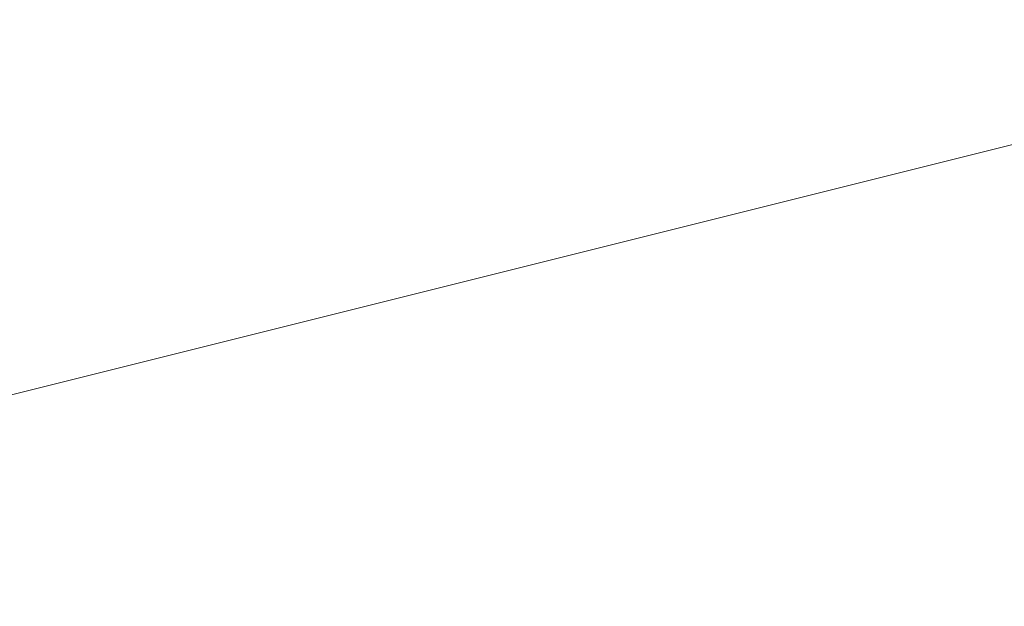
# Model space of a CAD drawing. Units: inches. Extents: x 2091 to 2899, y 967 to 2217.
# Tile 101 of 256: x 2252.3817 to 2252.951, y 1100.0709 to 1100.4099. Entities that reach past the tile are written whole.
import ezdxf

# ---------------------------------------------------------------- set-up
doc = ezdxf.new("R2010")
doc.units = ezdxf.units.IN
doc.layers.add('A-ANNO-DIMS', color=2, linetype='Continuous', lineweight=18)
doc.layers.add('L-PLNT-TREE', color=94, linetype='Continuous', lineweight=13)
doc.layers.add('A-WALL-PATT', color=141, linetype='Continuous', lineweight=13, true_color=0xadddf7)
doc.styles.get("Standard").update_dxf_attribs({"font": 'arial.ttf'})
doc.dimstyles.new('ISO-25', dxfattribs={"dimtxt": 4, "dimasz": 4, "dimexe": 1.25, "dimexo": 0.625, "dimtad": 1, "dimdec": 0, "dimlunit": 3, "dimtxsty": 'Standard', "dimcen": 2.5, "dimadec": 0, "dimazin": 0, "dimtfac": 1, "dimtdec": 0, "dimtmove": 0, "dimatfit": 3, "dimfxl": 1, "dimarcsym": 0})

# ---------------------------------------------------------------- blocks, each defined once
blk = doc.blocks.new('*U29')
blk.add_line((-402.336, 12.192), (-451.104, 0))
blk = doc.blocks.new('*D71')
at = {"layer": 'A-ANNO-DIMS', "color": 0, "lineweight": -2, "transparency": 16777216}
for p, q in [((2212.1436, 1351.29406), (2212.1436, 969.4643)), ((2452.1436, 1351.29406), (2452.1436, 969.4643)), ((2216.1436, 970.7143), (2448.1436, 970.7143))]:
    blk.add_line(p, q, dxfattribs=at)
at = {"layer": 'A-ANNO-DIMS', "color": 0, "transparency": 16777216}
for points in [[(2216.1436, 971.38097), (2216.1436, 970.04764), (2212.1436, 970.7143)], [(2448.1436, 971.38097), (2448.1436, 970.04764), (2452.1436, 970.7143)]]:
    blk.add_solid(points, dxfattribs=at)
at = {"layer": 'Defpoints', "color": 0, "transparency": 16777216}
for p in [(2212.1436, 1351.91906), (2452.1436, 1351.91906), (2452.1436, 970.7143)]:
    blk.add_point(p, dxfattribs=at)
at = {"layer": 'A-ANNO-DIMS', "color": 0, "transparency": 16777216, "insert": (2332.1436, 973.38159), "char_height": 4, "attachment_point": 5}
blk.add_mtext('20\'-0"', dxfattribs=at)
blk = doc.blocks.new('*D75')
at = {"layer": 'A-ANNO-DIMS', "color": 0, "lineweight": -2, "transparency": 16777216}
for p, q in [((2212.1436, 1274.79406), (2212.1436, 969.4643)), ((2308.1436, 1274.79406), (2308.1436, 969.4643)), ((2216.1436, 970.7143), (2304.1436, 970.7143))]:
    blk.add_line(p, q, dxfattribs=at)
at = {"layer": 'A-ANNO-DIMS', "color": 0, "transparency": 16777216}
for points in [[(2216.1436, 971.38097), (2216.1436, 970.04764), (2212.1436, 970.7143)], [(2304.1436, 971.38097), (2304.1436, 970.04764), (2308.1436, 970.7143)]]:
    blk.add_solid(points, dxfattribs=at)
at = {"layer": 'Defpoints', "color": 0, "transparency": 16777216}
for p in [(2212.1436, 1275.41906), (2308.1436, 1275.41906), (2308.1436, 970.7143)]:
    blk.add_point(p, dxfattribs=at)
at = {"layer": 'A-ANNO-DIMS', "color": 0, "transparency": 16777216, "insert": (2260.1436, 973.38159), "char_height": 4, "attachment_point": 5}
blk.add_mtext('8\'-0"', dxfattribs=at)

msp = doc.modelspace()

# ---------------------------------------------------------------- hatches: boundary and pattern name
at = {"layer": 'A-WALL-PATT'}
h = msp.add_hatch(color=256, dxfattribs=at)
h.dxf.hatch_style = 1
h.paths.add_polyline_path([(2803.1436, 2050.91906), (2203.1436, 2050.91906), (2203.1436, 1090.91906), (2803.1436, 1090.91906)])
h.paths.add_polyline_path([(2635.79885, 1147.54046), (2674.52405, 1147.54046, 0.376086), (2678.52967, 1152.8802), (2678.52967, 1159.55647, 0.333335), (2674.52432, 1163.56185), (2674.52432, 1163.56185), (2674.52432, 1192.93439), (2635.80597, 1192.93439), (2597.08762, 1192.93439), (2597.08762, 1163.56185, 0.333335), (2593.08228, 1159.55647), (2593.08228, 1152.8802, 0.376086), (2597.08789, 1147.54046)], flags=0)
h.paths.add_polyline_path([(2436.01043, 1278.24078, 0.000483), (2435.95264, 1278.21503, -0.001328), (2435.93563, 1278.11169, -0.001711), (2436.11644, 1278.04076, 0.002185)], flags=0)
h.paths.add_polyline_path([(2794.1436, 1143.41906), (2794.1436, 1347.41906), (2543.37017, 1347.41906), (2543.37017, 1351.91906), (2794.1436, 1351.91906), (2794.1436, 1392.71355), (2793.9474, 1392.71355), (2793.9474, 1473.5369), (2794.1436, 1473.5369), (2794.1436, 1531.91906), (2650.1436, 1531.91906), (2650.1436, 1536.41906), (2794.1436, 1536.41906), (2794.1436, 1692.41906), (2609.37561, 1692.41906), (2609.37561, 1644.41906), (2604.87561, 1644.41906), (2604.87561, 1744.91906), (2609.37561, 1744.91906), (2609.37561, 1696.91906), (2794.1436, 1696.91906), (2794.1436, 1780.91906), (2609.6436, 1780.91906), (2493.87561, 1780.91906), (2493.87561, 1785.41906), (2609.6436, 1785.41906), (2794.1436, 1785.41906), (2794.1436, 1847.93882), (2793.95122, 1847.93882), (2793.95122, 1928.76217), (2794.1436, 1928.76217), (2794.1436, 1941.41906), (2614.1436, 1941.41906), (2614.1436, 1821.41906), (2609.6436, 1821.41906), (2609.6436, 1941.41906), (2392.1436, 1941.41906), (2392.1436, 1819.91906), (2387.6436, 1819.91906), (2387.6436, 1941.41906), (2212.1436, 1941.41906), (2212.1436, 1783.91906), (2392.1436, 1783.91906), (2392.1436, 1780.91906), (2212.1436, 1780.91906), (2212.1436, 1629.41906), (2387.6436, 1629.41906), (2387.6436, 1744.91906), (2392.1436, 1744.91906), (2392.1436, 1627.91906), (2317.1436, 1627.91906), (2317.1436, 1551.41906), (2317.1436, 1536.41906), (2459.38359, 1536.41906), (2459.38359, 1602.39648), (2463.88359, 1602.39648), (2463.88359, 1531.91906), (2456.6436, 1531.91906), (2456.6436, 1529.91906), (2452.1436, 1529.91906), (2452.1436, 1531.91906), (2312.6436, 1531.91906), (2312.6436, 1551.41906), (2306.1436, 1551.41906), (2306.1436, 1555.91906), (2308.1436, 1555.91906), (2308.1436, 1551.41906), (2312.6436, 1551.41906), (2312.6436, 1627.91906), (2212.1436, 1627.91906), (2212.1436, 1555.91906), (2270.1436, 1555.91906), (2270.1436, 1551.41906), (2212.1436, 1551.41906), (2212.1436, 1351.91906), (2272.1436, 1351.91906), (2272.1436, 1347.41906), (2212.1436, 1347.41906), (2212.1436, 1275.41906), (2308.1436, 1275.41906), (2308.1436, 1351.91906), (2452.1436, 1351.91906), (2452.1436, 1493.91906), (2456.6436, 1493.91906), (2456.6436, 1347.41906), (2312.6436, 1347.41906), (2312.6436, 1270.91906), (2212.1436, 1270.91906), (2212.1436, 1099.91906), (2281.23752, 1099.91906), (2282.87104, 1110.9138), (2282.00834, 1116.9966), (2278.55774, 1121.4204), (2268.20564, 1128.0562), (2272.08764, 1128.0562), (2273.81294, 1131.927), (2279.42034, 1134.6919), (2285.02784, 1135.2449), (2287.61584, 1137.4568), (2288.04714, 1138.0098), (2289.34114, 1140.7747), (2291.06654, 1139.6687), (2292.36054, 1135.2449), (2295.37984, 1136.9038), (2296.24254, 1135.7979), (2297.10524, 1133.033), (2300.12464, 1138.0098), (2303.14394, 1138.0098), (2304.43794, 1135.7979), (2303.14394, 1133.586), (2306.59464, 1134.6919), (2307.88874, 1133.033), (2310.90804, 1135.2449), (2313.92744, 1134.1389), (2315.62686, 1132.4271), (2308.32004, 1117.5496), (2290.20384, 1109.8079), (2288.90984, 1103.1721), (2289.27231, 1099.91906), (2434.91823, 1099.91906), (2431.59323, 1124.78806), (2429.93023, 1169.55306), (2430.92718, 1240.51969), (2435.65893, 1238.18613), (2437.13523, 1196.55406), (2438.79823, 1143.97306), (2442.67823, 1111.99806), (2446.55823, 1099.91906), (2794.1436, 1099.91906), (2794.1436, 1138.91906), (2548.03245, 1138.91906), (2548.03245, 1143.41906), (2548.03245, 1148.81906), (2546.66846, 1148.03156), (2528.68569, 1179.17862, 0.256256), (2512.03245, 1148.81906), (2512.03245, 1143.41906), (2512.03245, 1138.91906), (2507.53245, 1138.91906), (2507.53245, 1143.41906), (2507.53245, 1148.81906, 0.256256), (2490.8792, 1179.17862), (2472.89644, 1148.03156), (2471.53245, 1148.81906), (2471.53245, 1143.41906), (2467.03245, 1143.41906), (2467.03245, 1269.94579, 0.039061), (2460.90999, 1273.58006), (2467.03245, 1273.58006), (2467.03245, 1286.32536, 0.014511), (2465.21619, 1286.76191), (2467.03245, 1287.05258), (2467.03245, 1323.41906), (2471.53245, 1323.41906), (2471.53245, 1148.81906), (2489.53245, 1179.99597), (2490.89644, 1179.20847), (2490.8792, 1179.17862, -0.256256), (2507.53245, 1148.81906), (2507.53245, 1143.41906), (2512.03245, 1143.41906), (2512.03245, 1148.81906, -0.256256), (2528.68569, 1179.17862), (2528.66846, 1179.20847), (2530.03245, 1179.99597), (2548.03245, 1148.81906), (2548.03245, 1143.41906)], flags=16)
h.paths.add_polyline_path([(2607.76855, 1200.94508), (2607.76855, 1265.03063), (2597.08762, 1281.05201), (2619.78459, 1281.05201), (2627.79528, 1337.12686), (2635.79885, 1337.12686), (2643.81666, 1337.12686), (2651.82736, 1281.05201), (2674.52432, 1281.05201), (2663.8434, 1265.03063), (2663.8434, 1200.94508), (2635.80597, 1200.94508)], flags=0)
edge = h.paths.add_edge_path(flags=0)
edge.add_ellipse((13303.89622, 1272.99872), major_axis=(-10595.31304, 0), ratio=0.84230387009, start_angle=0.628237219, end_angle=0.6465541, ccw=False)
edge.add_ellipse((2711.70045, 1156.85268), major_axis=(2.21977, 0), ratio=0.8423039, start_angle=111.53524, end_angle=180.62824, ccw=False)
edge.add_ellipse((13303.15629, 1272.99872), major_axis=(-10593.02631, 0), ratio=0.84230386954, start_angle=0.528271472, end_angle=0.646554097, ccw=False)
edge.add_line((2710.7646, 1175.3333), (2710.12999, 1175.3333))
edge.add_ellipse((2710.12999, 1176.57978), major_axis=(1.47985, 0), ratio=0.8423039, start_angle=180, end_angle=270, ccw=False)
edge.add_line((2708.65014, 1176.57978), (2708.65014, 1200.78291))
edge.add_ellipse((2710.12999, 1200.78291), major_axis=(1.47985, 0), ratio=0.8423039, start_angle=90, end_angle=180, ccw=False)
edge.add_line((2710.12999, 1202.02939), (2710.46508, 1202.02939))
edge.add_ellipse((13303.15629, 1272.99872), major_axis=(-10593.02631, 0), ratio=0.84230386954, start_angle=-0.090229089, end_angle=0.383866779, ccw=False)
edge.add_ellipse((2710.12999, 1290.92703), major_axis=(-1.47985, 0), ratio=0.8423039, start_angle=0, end_angle=90, ccw=False)
edge.add_line((2708.65014, 1290.92703), (2708.65014, 1315.13017))
edge.add_ellipse((2710.12999, 1315.13017), major_axis=(-1.47985, 0), ratio=0.8423039, start_angle=-90, end_angle=0, ccw=False)
edge.add_line((2710.12999, 1316.37665), (2710.70631, 1316.37665))
edge.add_ellipse((3238.40172, 1296.28957), major_axis=(528.234, 0), ratio=0.84230387, start_angle=176.3495724, end_angle=177.8200497, ccw=False)
edge.add_ellipse((2775.06304, 1071.4507), major_axis=(313.30776, 0), ratio=0.84230387, start_angle=102.1259656, end_angle=103.780529, ccw=False)
edge.add_ellipse((2775.06304, 1078.3057), major_axis=(-305.30289, 0), ratio=0.84230387, start_angle=-79.790461, end_angle=-77.5553727, ccw=False)
edge.add_ellipse((2695.14177, 1541.97538), major_axis=(-250.96022, 0), ratio=0.84230387, start_angle=99.256566, end_angle=102.5549326)
edge.add_line((2741.41033, 1334.21426), (2747.13255, 1337.37848))
edge.add_ellipse((2747.53862, 1336.85748), major_axis=(-0.73992, 0), ratio=0.842304, start_angle=270, end_angle=307.93313, ccw=False)
edge.add_ellipse((2747.53862, 1336.85748), major_axis=(-0.73992, 0), ratio=0.842304, start_angle=232.06687, end_angle=270, ccw=False)
edge.add_line((2747.94469, 1337.37848), (2753.66691, 1334.21426))
edge.add_ellipse((2799.93547, 1541.97538), major_axis=(250.96022, 0), ratio=0.84230387, start_angle=257.4450674, end_angle=260.743434)
edge.add_ellipse((2720.01419, 1078.3057), major_axis=(305.30289, 0), ratio=0.84230387, start_angle=77.5553727, end_angle=79.790461, ccw=False)
edge.add_ellipse((2720.01419, 1071.4507), major_axis=(-313.30776, 0), ratio=0.84230387, start_angle=256.219471, end_angle=257.8740344, ccw=False)
edge.add_ellipse((2256.67551, 1296.28957), major_axis=(-528.234, 0), ratio=0.84230387, start_angle=182.1799503, end_angle=183.6504276, ccw=False)
edge.add_line((2784.37092, 1316.37665), (2784.94725, 1316.37665))
edge.add_ellipse((2784.94725, 1315.13017), major_axis=(1.47985, 0), ratio=0.8423039, start_angle=0, end_angle=90, ccw=False)
edge.add_line((2786.42709, 1315.13017), (2786.42709, 1290.92703))
edge.add_ellipse((2784.94725, 1290.92703), major_axis=(1.47985, 0), ratio=0.8423039, start_angle=270, end_angle=360, ccw=False)
edge.add_ellipse((-7808.07906, 1272.99872), major_axis=(10593.02631, 0), ratio=0.84230386954, start_angle=-0.383866779, end_angle=0.090229089, ccw=False)
edge.add_line((2784.61216, 1202.02939), (2784.94725, 1202.02939))
edge.add_ellipse((2784.94725, 1200.78291), major_axis=(1.47985, 0), ratio=0.8423039, start_angle=0, end_angle=90, ccw=False)
edge.add_line((2786.42709, 1200.78291), (2786.42709, 1176.57978))
edge.add_ellipse((2784.94725, 1176.57978), major_axis=(-1.47985, 0), ratio=0.8423039, start_angle=90, end_angle=180, ccw=False)
edge.add_line((2784.94725, 1175.3333), (2784.31264, 1175.3333))
edge.add_ellipse((-7808.07906, 1272.99872), major_axis=(10593.02631, 0), ratio=0.84230386954, start_angle=-0.618643196, end_angle=-0.528271472, ccw=False)
edge.add_ellipse((2783.37678, 1156.85268), major_axis=(-2.21977, 0), ratio=0.8423039, start_angle=179.37176, end_angle=248.46476, ccw=False)
edge.add_ellipse((-7808.81898, 1272.99872), major_axis=(-10595.31304, 0), ratio=0.84230386576, start_angle=179.353445923, end_angle=179.371762803, ccw=False)
edge.add_ellipse((2780.2973, 1153.50079), major_axis=(-5.24643, 0), ratio=0.8423039, start_angle=90, end_angle=179.35345, ccw=False)
edge.add_line((2780.2973, 1149.08171), (2714.77993, 1149.08171))
edge.add_ellipse((2714.77993, 1153.50079), major_axis=(5.24643, 0), ratio=0.8423039, start_angle=180.64655, end_angle=270, ccw=False)
edge = h.paths.add_edge_path(flags=0)
edge.add_line((2718.18737, 1151.00783), (2718.18737, 1170.47236))
edge.add_ellipse((2721.14706, 1170.47236), major_axis=(-2.95969, 0), ratio=0.8423039, start_angle=-90, end_angle=0, ccw=False)
edge.add_line((2721.14706, 1172.96532), (2773.93017, 1172.96532))
edge.add_ellipse((2773.93017, 1170.47236), major_axis=(-2.95969, 0), ratio=0.8423039, start_angle=180, end_angle=270, ccw=False)
edge.add_line((2776.88987, 1170.47236), (2776.88987, 1151.00783))
edge.add_line((2776.88987, 1151.00783), (2718.18737, 1151.00783))
edge = h.paths.add_edge_path(flags=0)
edge.add_line((2718.18737, 1180.23415), (2718.18737, 1199.05783))
edge.add_ellipse((2747.53862, 1320.39864), major_axis=(147.01792, 0), ratio=0.84230387, start_angle=256.4018653, end_angle=283.5981347)
edge.add_line((2776.88987, 1199.05783), (2776.88987, 1180.23415))
edge.add_ellipse((2747.53862, 1301.57496), major_axis=(147.01792, 0), ratio=0.84230387, start_angle=256.4018653, end_angle=283.5981347, ccw=False)
edge = h.paths.add_edge_path(flags=0)
edge.add_ellipse((13303.15629, 1272.99872), major_axis=(-10591.54646, 0), ratio=0.84230386955, start_angle=0.055594314, end_angle=0.377764194, ccw=False)
edge.add_line((2711.61686, 1262.72171), (2715.66741, 1249.4954))
edge.add_ellipse((6413.89196, 1241.69192), major_axis=(-3698.23616, 0), ratio=0.8423038695, start_angle=-0.12089737, end_angle=0.36407635)
edge.add_line((2715.76104, 1218.19245), (2711.93431, 1203.16736))
edge = h.paths.add_edge_path(flags=0)
edge.add_line((2718.18737, 1251.07457), (2716.00249, 1267.45044))
edge.add_ellipse((2742.15117, 1202.18954), major_axis=(81.77258, 0), ratio=0.84230387, start_angle=94.277421, end_angle=111.8349538, ccw=False)
edge.add_line((2737.00975, 1270.93063), (2758.06748, 1270.93063))
edge.add_ellipse((2752.92606, 1202.18954), major_axis=(81.77258, 0), ratio=0.84230387, start_angle=68.1650462, end_angle=85.722579, ccw=False)
edge.add_line((2779.07475, 1267.45044), (2776.88987, 1251.07457))
edge.add_ellipse((2750.33806, 1187.88536), major_axis=(79.57966, 0), ratio=0.84230387, start_angle=67.2080851, end_angle=85.1299304)
edge.add_line((2756.03466, 1254.74366), (2739.04258, 1254.74366))
edge.add_ellipse((2744.73917, 1187.88536), major_axis=(79.57966, 0), ratio=0.84230387, start_angle=94.8700696, end_angle=112.7919149)
edge = h.paths.add_edge_path(flags=0)
edge.add_line((2783.14293, 1203.16736), (2779.31619, 1218.19245))
edge.add_ellipse((-918.81473, 1241.69192), major_axis=(3698.23616, 0), ratio=0.8423038695, start_angle=-0.36407635, end_angle=0.12089737)
edge.add_line((2779.40983, 1249.4954), (2783.46037, 1262.72171))
edge.add_ellipse((-7808.07906, 1272.99872), major_axis=(-10591.54646, 0), ratio=0.84230386954, start_angle=179.622235806, end_angle=179.944405687, ccw=False)
edge = h.paths.add_edge_path(flags=0)
edge.add_ellipse((2734.20089, 1286.69044), major_axis=(-0.35661, 6.34008), ratio=0.6038336, start_angle=89.002014, end_angle=253.657408, ccw=False)
edge.add_line((2730.369, 1286.54181), (2730.369, 1301.35198))
edge.add_line((2730.369, 1301.35198), (2735.91331, 1305.2148))
edge.add_ellipse((2736.38492, 1304.73456), major_axis=(0.73992, 0), ratio=0.842304, start_angle=90, end_angle=134.48021, ccw=False)
edge.add_line((2736.38492, 1305.3578), (2738.03278, 1305.3578))
edge.add_line((2738.03278, 1305.3578), (2738.03278, 1307.70793))
edge.add_ellipse((2794.20164, 1307.70793), major_axis=(56.16886, 0), ratio=0.84230387, start_angle=150.56143, end_angle=180, ccw=False)
edge.add_ellipse((2700.87559, 1307.70793), major_axis=(-56.16886, 0), ratio=0.84230387, start_angle=180, end_angle=209.43857, ccw=False)
edge.add_line((2757.04445, 1307.70793), (2757.04445, 1305.3578))
edge.add_line((2757.04445, 1305.3578), (2758.69232, 1305.3578))
edge.add_ellipse((2758.69232, 1304.73456), major_axis=(-0.73992, 0), ratio=0.842304, start_angle=225.51979, end_angle=270, ccw=False)
edge.add_line((2759.16392, 1305.2148), (2764.70823, 1301.35198))
edge.add_line((2764.70823, 1301.35198), (2764.70823, 1286.54181))
edge.add_ellipse((2760.87634, 1286.69044), major_axis=(0.35661, 6.34008), ratio=0.6038336, start_angle=106.342592, end_angle=270.997986, ccw=False)
edge.add_line((2757.04445, 1285.79709), (2757.04445, 1307.70793))
edge.add_ellipse((2700.87559, 1307.70793), major_axis=(-56.16886, 0), ratio=0.84230387, start_angle=180, end_angle=209.43857)
edge.add_ellipse((2794.20164, 1307.70793), major_axis=(56.16886, 0), ratio=0.84230387, start_angle=150.56143, end_angle=180)
edge.add_line((2738.03278, 1307.70793), (2738.03278, 1285.79709))
h.paths.add_polyline_path([(2417.81227, 1104.4497), (2413.49227, 1102.5297), (2410.61227, 1103.9697), (2409.17227, 1106.3697), (2407.25227, 1107.3297), (2406.29227, 1109.7297), (2405.33227, 1114.0497), (2405.33227, 1117.8897), (2406.29227, 1120.1297), (2407.25227, 1119.8097), (2408.84832, 1118.32766), (2410.17395, 1119.42417), (2410.21127, 1120.4057), (2411.04073, 1121.41905), (2410.69927, 1119.8587), (2410.17395, 1119.42417), (2410.08845, 1117.17611), (2411.13284, 1116.20632), (2413.97227, 1119.3297), (2416.85227, 1120.7697), (2416.86972, 1120.79878), (2417.03507, 1119.40512), (2417.89621, 1118.14338), (2418.29227, 1118.3697), (2419.54445, 1120.03927), (2419.36092, 1118.38749), (2419.03211, 1119.35615), (2418.39894, 1118.51193), (2419.25227, 1114.5297), (2418.79409, 1107.19879)], flags=0)
h.paths.add_polyline_path([(2508.87017, 1347.41906), (2508.37017, 1347.41906), (2508.37017, 1351.91906), (2508.87017, 1351.91906)], flags=0)
h.paths.add_polyline_path([(2473.37017, 1347.41906), (2472.37017, 1347.41906), (2467.87017, 1347.41906), (2467.87017, 1455.41906), (2472.37017, 1455.41906), (2472.37017, 1352.41906), (2473.37017, 1352.41906)], flags=0)
h.paths.add_polyline_path([(2352.10624, 1217.4462), (2349.22624, 1218.8862), (2347.78624, 1221.2862), (2345.86624, 1222.2462), (2344.90624, 1224.6462), (2343.94624, 1228.9662), (2343.94624, 1232.8062), (2344.90624, 1235.0462), (2345.86624, 1234.7262), (2347.46229, 1233.24415), (2348.78792, 1234.34066), (2348.82524, 1235.3222), (2349.6547, 1236.33555), (2349.31324, 1234.7752), (2348.78792, 1234.34066), (2348.70242, 1232.0926), (2349.74681, 1231.12282), (2352.58624, 1234.2462), (2355.46624, 1235.6862), (2355.48369, 1235.71528), (2355.64904, 1234.32161), (2356.51018, 1233.05988), (2356.90624, 1233.2862), (2358.15842, 1234.95576), (2357.97489, 1233.30398), (2357.64608, 1234.27264), (2357.01291, 1233.42842), (2357.86624, 1229.4462), (2357.40806, 1222.11529), (2356.42624, 1219.3662)], flags=0)
h.paths.add_polyline_path([(2348.2968, 1112.22442), (2347.0138, 1112.31042), (2345.5298, 1114.12742), (2345.7318, 1115.85842), (2346.8118, 1116.98242), (2346.8118, 1114.64642), (2345.8668, 1114.21442), (2346.8798, 1114.30042)], flags=0)
h.paths.add_polyline_path([(2347.0138, 1110.92642), (2346.2718, 1110.49342), (2346.6098, 1111.18642)], flags=0)
h.paths.add_polyline_path([(2345.8668, 1118.19442), (2345.5298, 1117.32942), (2343.7078, 1118.02142), (2344.3828, 1118.62642)], flags=0)
h.paths.add_polyline_path([(2346.6768, 1109.28242), (2346.0698, 1108.07142), (2345.8668, 1110.06142)], flags=0)
h.paths.add_polyline_path([(2345.0568, 1119.75142), (2343.6398, 1119.75142), (2343.9778, 1121.13542)], flags=0)
h.paths.add_polyline_path([(2345.2598, 1116.55042), (2345.1248, 1115.85842), (2344.9218, 1115.68542), (2344.7198, 1116.37742)], flags=0)
h.paths.add_polyline_path([(2345.6648, 1112.31042), (2345.4618, 1111.53242), (2344.0448, 1111.96442), (2344.6518, 1112.57042)], flags=0)
h.paths.add_polyline_path([(2345.1918, 1113.34942), (2344.4498, 1113.86842), (2344.7198, 1114.38742)], flags=0)
h.paths.add_polyline_path([(2344.6518, 1116.80942), (2344.1798, 1115.68542), (2344.6518, 1115.33942), (2343.9098, 1114.90642), (2343.0328, 1115.94442), (2343.6398, 1116.46342)], flags=0)
h.paths.add_polyline_path([(2345.8668, 1106.68642), (2344.9898, 1105.56242), (2344.5168, 1106.60042)], flags=0)
h.paths.add_polyline_path([(2344.8548, 1110.06142), (2344.5168, 1109.28242), (2344.1128, 1109.71542)], flags=0)
h.paths.add_polyline_path([(2344.0448, 1113.52242), (2343.4378, 1113.08942), (2342.7628, 1113.95442)], flags=0)
h.paths.add_polyline_path([(2344.3148, 1111.01242), (2342.9648, 1110.32042), (2342.9648, 1111.09942)], flags=0)
h.paths.add_polyline_path([(2345.1248, 1104.69742), (2344.5848, 1103.74542), (2344.4498, 1104.26442)], flags=0)
h.paths.add_polyline_path([(2342.8298, 1121.22242), (2341.7498, 1120.53042), (2340.5358, 1121.04942), (2340.1308, 1121.82842), (2340.6708, 1122.95242), (2341.1428, 1121.82842), (2341.6148, 1122.00142)], flags=0)
h.paths.add_polyline_path([(2342.9648, 1119.75142), (2343.0328, 1118.45342), (2342.0878, 1118.02142), (2342.0198, 1119.49142)], flags=0)
h.paths.add_polyline_path([(2342.6948, 1116.89642), (2341.9528, 1116.63642), (2342.0198, 1117.32942)], flags=0)
h.paths.add_polyline_path([(2343.0328, 1112.22442), (2342.0198, 1111.79142), (2341.5478, 1112.22442), (2342.3578, 1113.34942)], flags=0)
h.paths.add_polyline_path([(2343.7748, 1104.43742), (2342.6278, 1102.88042), (2342.6948, 1104.61042), (2343.4378, 1105.12942)], flags=0)
h.paths.add_polyline_path([(2342.0198, 1115.07942), (2340.8058, 1115.51242), (2340.9408, 1116.37742)], flags=0)
h.paths.add_polyline_path([(2341.4808, 1120.09742), (2341.4808, 1119.40542), (2341.0758, 1119.57842), (2341.1428, 1120.09742)], flags=0)
h.paths.add_polyline_path([(2341.8178, 1114.47342), (2340.9408, 1113.08942), (2340.8058, 1114.56042)], flags=0)
h.paths.add_polyline_path([(2341.1428, 1118.54042), (2340.9408, 1116.98242), (2339.0508, 1117.67542), (2339.0508, 1118.62642)], flags=0)
h.paths.add_polyline_path([(2342.6948, 1101.66842), (2341.9528, 1101.84142), (2342.5598, 1102.36142)], flags=0)
h.paths.add_polyline_path([(2340.3328, 1119.66542), (2338.4438, 1119.57842), (2337.9038, 1120.35742), (2339.6578, 1120.61642)], flags=0)
h.paths.add_polyline_path([(2340.3328, 1115.33942), (2340.0628, 1113.69542), (2339.3878, 1115.33942)], flags=0)
h.paths.add_polyline_path([(2341.8178, 1103.83142), (2341.5478, 1102.88042), (2341.1428, 1103.65842)], flags=0)
h.paths.add_polyline_path([(2339.0508, 1122.86642), (2337.2958, 1121.82842), (2337.0938, 1123.12542), (2337.7688, 1123.81842)], flags=0)
h.paths.add_polyline_path([(2339.1178, 1121.74142), (2338.8478, 1121.22242), (2338.1738, 1121.04942), (2338.3758, 1121.56842)], flags=0)
h.paths.add_polyline_path([(2339.1858, 1119.31942), (2338.6458, 1118.71342), (2338.2408, 1118.10742), (2338.2408, 1118.88642)], flags=0)
h.paths.add_polyline_path([(2341.1428, 1101.92842), (2340.6028, 1101.23642), (2340.0628, 1101.84142), (2340.6028, 1102.36142)], flags=0)
h.paths.add_polyline_path([(2337.6338, 1117.76142), (2336.6208, 1118.28042), (2337.2958, 1118.97242)], flags=0)
h.paths.add_polyline_path([(2336.8238, 1119.57842), (2334.7988, 1118.97242), (2335.2038, 1120.35742), (2336.5538, 1120.87642)], flags=0)
h.paths.add_polyline_path([(2339.1178, 1100.45742), (2337.3638, 1100.54342), (2336.7558, 1101.23642)], flags=0)
h.paths.add_polyline_path([(2336.3508, 1122.43342), (2336.0138, 1121.91442), (2334.9338, 1122.43342), (2334.5288, 1123.47142), (2335.7438, 1122.77942)], flags=0)
h.paths.add_polyline_path([(2334.7318, 1120.87642), (2334.2588, 1120.35742), (2334.0568, 1120.78942), (2334.5968, 1121.30842)], flags=0)
h.paths.add_polyline_path([(2334.4618, 1122.17442), (2332.5718, 1121.30842), (2331.3568, 1122.17442), (2332.0998, 1122.86642)], flags=0)
h.paths.add_polyline_path([(2334.2588, 1118.54042), (2333.3818, 1118.45342), (2333.6518, 1119.31942)], flags=0)
h.paths.add_polyline_path([(2335.5418, 1102.27442), (2334.1918, 1102.62042), (2335.2718, 1103.31242)], flags=0)
h.paths.add_polyline_path([(2332.7068, 1119.66542), (2331.6948, 1120.44342), (2332.5048, 1120.78942)], flags=0)
h.paths.add_polyline_path([(2334.7318, 1101.14942), (2333.5168, 1101.58242), (2333.9888, 1101.75542)], flags=0)
h.paths.add_polyline_path([(2332.6398, 1116.63642), (2331.0868, 1116.29042), (2331.9648, 1118.19442)], flags=0)
h.paths.add_polyline_path([(2330.7498, 1121.56842), (2330.2768, 1120.27042), (2328.5228, 1119.31942), (2328.9948, 1121.04942)], flags=0)
h.paths.add_polyline_path([(2330.7498, 1118.62642), (2330.0078, 1117.50242), (2329.8728, 1118.02142)], flags=0)
h.paths.add_polyline_path([(2332.0998, 1102.36142), (2330.5468, 1102.01442), (2331.6948, 1102.96642)], flags=0)
h.paths.add_polyline_path([(2329.5348, 1113.60842), (2329.0628, 1112.31042), (2328.5898, 1113.34942)], flags=0)
h.paths.add_polyline_path([(2328.3878, 1117.84842), (2327.5098, 1116.55042), (2327.1728, 1117.76142)], flags=0)
h.paths.add_polyline_path([(2329.7378, 1106.51342), (2329.5348, 1105.30242), (2328.2528, 1106.08142)], flags=0)
h.paths.add_polyline_path([(2328.6578, 1114.38742), (2328.0498, 1114.12742), (2328.3198, 1114.90642)], flags=0)
h.paths.add_polyline_path([(2328.3198, 1112.22442), (2327.1058, 1112.13742), (2326.7008, 1112.65642)], flags=0)
h.paths.add_polyline_path([(2326.9028, 1115.25242), (2326.7008, 1114.12742), (2325.2158, 1113.60842), (2326.0928, 1115.33942)], flags=0)
h.paths.add_polyline_path([(2326.6328, 1108.33042), (2326.0928, 1107.37942), (2325.8908, 1108.50342), (2326.4978, 1109.10942)], flags=0)
h.paths.add_polyline_path([(2615.1436, 1531.91906), (2609.6436, 1531.91906), (2609.6436, 1620.41906), (2614.1436, 1620.41906), (2614.1436, 1536.41906), (2615.1436, 1536.41906)], flags=0)
h.paths.add_polyline_path([(2545.1436, 1563.41906), (2464.1436, 1563.41906), (2464.1436, 1632.41906), (2509.1436, 1632.41906), (2509.1436, 1627.91906), (2509.1436, 1603.91906), (2468.6436, 1603.91906), (2468.6436, 1567.91906), (2540.6436, 1567.91906), (2540.6436, 1591.91906), (2545.1436, 1591.91906)], flags=0)
h.paths.add_polyline_path([(2388.96905, 1549.98573), (2357.43418, 1549.98573), (2357.43418, 1623.36078), (2399.36278, 1623.36078), (2435.68947, 1623.36078), (2435.59255, 1602.55927), (2435.59255, 1602.39648), (2388.96905, 1602.39648)], flags=0)
h.paths.add_polyline_path([(2388.88063, 1555.80915), (2374.90443, 1555.80915), (2374.90443, 1600.57156), (2374.90443, 1615.45765), (2406.35088, 1615.45765), (2406.35088, 1618.93943), (2412.17429, 1615.45765), (2406.35088, 1611.97586), (2406.35088, 1615.45765), (2388.88063, 1615.45765)], flags=0)
h.paths.add_polyline_path([(2568.87561, 1644.41906), (2453.37561, 1644.41906), (2453.37561, 1785.41906), (2457.87561, 1785.41906), (2457.87561, 1648.91906), (2568.87561, 1648.91906)], flags=0)
h.paths.add_polyline_path([(2212.1436, 1945.91906), (2212.1436, 2041.91906), (2794.1436, 2041.91906), (2794.1436, 1945.91906)], flags=16)
h.paths.add_polyline_path([(2271.08273, 1964.31724), (2776.85297, 1964.31724), (2776.85297, 2037.16962), (2271.08273, 2037.16962)], flags=8)
h.paths.add_polyline_path([(2380.64929, 1536.82414), (2461.04081, 1536.82414), (2461.04081, 1554.65259), (2380.64929, 1554.65259)], flags=8)
h.paths.add_polyline_path([(2240.75571, 1609.72545), (2309.18583, 1609.72545), (2309.18583, 1617.6982), (2240.75571, 1617.6982)], flags=8)
h.paths.add_polyline_path([(2212.67726, 1313.5041), (2282.59152, 1313.5041), (2282.59152, 1322.74524), (2212.67726, 1322.74524)], flags=8)
h.paths.add_polyline_path([(2457.11198, 1114.77857), (2558.48158, 1114.77857), (2558.48158, 1142.21968), (2457.11198, 1142.21968)], flags=8)
h.paths.add_polyline_path([(2473.44234, 1273.01007), (2604.64123, 1273.01007), (2604.64123, 1318.34693), (2473.44234, 1318.34693)], flags=8)
h.paths.add_polyline_path([(2638.8763, 1626.97743), (2684.25037, 1627.97674), (2684.03848, 1637.59749), (2638.66442, 1636.59819)], flags=8)
h.paths.add_polyline_path([(2537.59055, 1453.79345), (2628.38955, 1453.79345), (2628.38955, 1475.34481), (2537.59055, 1475.34481)], flags=8)
h.paths.add_polyline_path([(2504.13764, 1714.6324), (2554.64719, 1714.6324), (2554.64719, 1730.23771), (2504.13764, 1730.23771)], flags=8)
h.paths.add_polyline_path([(2487.50118, 1575.65187), (2535.09712, 1575.65187), (2535.09712, 1598.37765), (2487.50118, 1598.37765)], flags=8)
h.paths.add_polyline_path([(2709.0994, 1735.71028), (2740.0166, 1735.71028), (2740.0166, 1749.93764), (2709.0994, 1749.93764)], flags=8)
h.paths.add_polyline_path([(2442.43842, 1792.17166), (2564.72884, 1792.17166), (2564.72884, 1842.00016), (2442.43842, 1842.00016)], flags=8)
h.paths.add_polyline_path([(2655.8158, 1809.64408), (2789.52014, 1806.6938), (2790.08498, 1832.29164), (2656.38064, 1835.24192)], flags=8)
h.paths.add_polyline_path([(2234.8427, 1797.72014), (2368.59285, 1794.76885), (2369.16072, 1820.50413), (2235.41056, 1823.45542)], flags=8)
h.paths.add_polyline_path([(2245.13847, 1644.00633), (2398.42773, 1640.6239), (2398.99484, 1666.32482), (2245.70557, 1669.70725)], flags=8)
h.paths.add_polyline_path([(2306.14285, 1431.16852), (2413.76831, 1428.79369), (2414.33315, 1454.39153), (2306.70768, 1456.76636)], flags=8)
h.paths.add_polyline_path([(2306.83458, 1458.23314), (2393.38048, 1456.32345), (2393.93281, 1481.35436), (2307.38691, 1483.26405)], flags=8)

# ---------------------------------------------------------------- block references
at = {"layer": 'L-PLNT-TREE', "xscale": 0.0393700787401575, "yscale": 0.0393700787401575, "zscale": 0.0393700787401575}
msp.add_blockref('*U29', (2269.04101, 1099.91906), dxfattribs=at)

# ---------------------------------------------------------------- dimensions: what is measured, and where the dimension line sits
at = {"layer": 'A-ANNO-DIMS'}
for base, p1, p2, picture, middle in [((2452.1436, 970.7143), (2212.1436, 1351.91906), (2452.1436, 1351.91906), '*D71', (2332.1436, 973.38159)), ((2308.1436, 970.7143), (2212.1436, 1275.41906), (2308.1436, 1275.41906), '*D75', (2260.1436, 973.38159))]:
    dim = msp.add_linear_dim(base=base, p1=p1, p2=p2, dimstyle='ISO-25', override={"dimdec": 1, "dimlfac": 1, "dimrnd": 0, "dimzin": 1, "dimdsep": 46, "dimlunit": 4, "dimfrac": 2}, dxfattribs=at)
    dim.commit()
    dim.dimension.update_dxf_attribs({"geometry": picture, "text_midpoint": middle})

doc.saveas('drawing.dxf')
